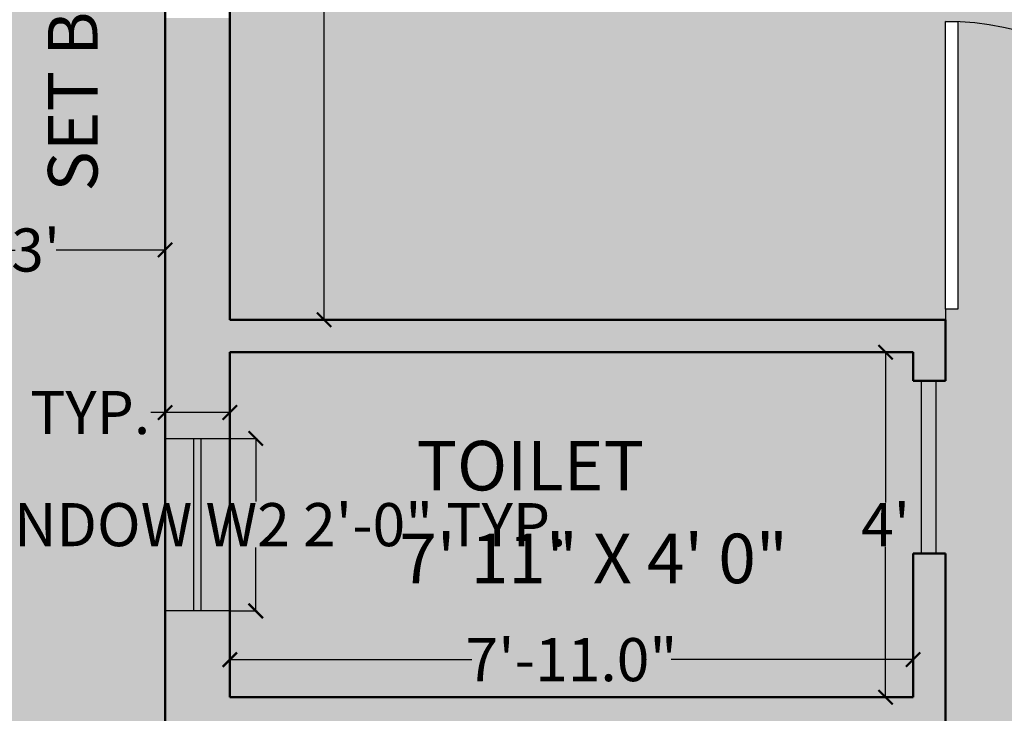
# Model space of a CAD drawing. Units: inches. Extents: x 528 to 2620, y -1066 to 798.
# Tile 6 of 41: x 600 to 737, y 523 to 620. Entities that reach past the tile are written whole.
import ezdxf

# ---------------------------------------------------------------- set-up
doc = ezdxf.new("R2010")
doc.units = ezdxf.units.IN
doc.header["$MEASUREMENT"] = 0
for name, color, linetype, lineweight in [('A-ANNO-DIMS', 2, 'Continuous', 18), ('A-AREA-IDEN', 7, 'Continuous', 18), ('A-Door', 2, 'Continuous', 25), ('A-GLAZ', 3, 'Continuous', 25), ('A-WALL', 7, 'Continuous', 50), ('A-WALL-PATT', 8, 'Continuous', 13)]:
    doc.layers.add(name, color=color, linetype=linetype, lineweight=lineweight)
doc.styles.get("Standard").update_dxf_attribs({"font": 'arial.ttf'})
doc.dimstyles.get("Standard").update_dxf_attribs({"dimtxt": 6, "dimasz": 2, "dimexe": 0.18, "dimexo": 0.0625, "dimgap": 0.09, "dimtad": 0, "dimtih": 1, "dimtoh": 1, "dimdec": 1, "dimzin": 0, "dimdsep": 46, "dimlunit": 3, "dimtxsty": 'Standard', "dimblk": 'ARCHTICK', "dimcen": 0.09, "dimadec": 0, "dimazin": 0, "dimtfac": 1, "dimtdec": 1, "dimtofl": 0, "dimtmove": 0, "dimatfit": 3, "dimfxl": 1, "dimtolj": 1, "dimtzin": 0, "dimarcsym": 0})

# ---------------------------------------------------------------- blocks, each defined once
blk = doc.blocks.new('*U4')
for p, q in [((0, 0), (0, -6)), ((40, 0), (40, -6))]:
    blk.add_line(p, q)
blk.add_lwpolyline([(0, 0), (0, 40), (1.75, 40), (1.75, 0)], close=True)
blk.add_arc((0, 0), 40, 0, 90)
blk = doc.blocks.new('_ArchTick')
at = {"color": 0, "linetype": 'ByBlock', "const_width": 0.15}
blk.add_lwpolyline([(-0.5, -0.5), (0.5, 0.5)], dxfattribs=at)
blk = doc.blocks.new('*D14')
at = {"layer": 'A-ANNO-DIMS', "color": 0, "lineweight": -2, "transparency": 16777216}
for p, q in [((584.06, 587.76), (584.06, 587.45)), ((584.06, 587.63), (599.21, 587.63)), ((620.06, 587.63), (604.91, 587.63)), ((620.06, 587.76), (620.06, 587.45))]:
    blk.add_line(p, q, dxfattribs=at)
at = {"layer": 'Defpoints', "color": 0, "transparency": 16777216}
for p in [(584.06, 587.82), (584.06, 587.63), (620.06, 587.82)]:
    blk.add_point(p, dxfattribs=at)
at = {"layer": 'A-ANNO-DIMS', "color": 0, "lineweight": -2, "transparency": 16777216, "xscale": 2, "yscale": 2, "zscale": 2, "rotation": 180}
blk.add_blockref('_ArchTick', (584.06, 587.63), dxfattribs=at)
at = {"layer": 'A-ANNO-DIMS', "color": 0, "lineweight": -2, "transparency": 16777216, "xscale": 2, "yscale": 2, "zscale": 2}
blk.add_blockref('_ArchTick', (620.06, 587.63), dxfattribs=at)
at = {"layer": 'A-ANNO-DIMS', "color": 0, "transparency": 16777216, "insert": (602.06, 587.63), "char_height": 6, "attachment_point": 5}
blk.add_mtext("\\A1;3'", dxfattribs=at)
blk = doc.blocks.new('*D26')
at = {"layer": 'A-ANNO-DIMS', "color": 0, "lineweight": -2, "transparency": 16777216}
for p, q in [((642.51, 709.92), (641.99, 709.92)), ((642.17, 709.92), (642.17, 647.02)), ((642.17, 577.92), (642.17, 640.82)), ((642.51, 577.92), (641.99, 577.92))]:
    blk.add_line(p, q, dxfattribs=at)
at = {"layer": 'Defpoints', "color": 0, "transparency": 16777216}
for p in [(642.57, 709.92), (642.17, 577.92), (642.57, 577.92)]:
    blk.add_point(p, dxfattribs=at)
at = {"layer": 'A-ANNO-DIMS', "color": 0, "lineweight": -2, "transparency": 16777216, "xscale": 2, "yscale": 2, "zscale": 2}
for p, rotation in [((642.17, 709.92), 90), ((642.17, 577.92), 270)]:
    blk.add_blockref('_ArchTick', p, dxfattribs=dict(at, rotation=rotation))
at = {"layer": 'A-ANNO-DIMS', "color": 0, "transparency": 16777216, "insert": (642.17, 643.92), "char_height": 6, "attachment_point": 5}
blk.add_mtext("\\A1;11'", dxfattribs=at)
blk = doc.blocks.new('*D31')
at = {"layer": 'A-ANNO-DIMS', "color": 0, "lineweight": -2, "transparency": 16777216}
for p, q in [((720.5, 573.42), (720.06, 573.42)), ((720.24, 573.42), (720.24, 552.51)), ((720.24, 525.42), (720.24, 546.33)), ((720.5, 525.42), (720.06, 525.42))]:
    blk.add_line(p, q, dxfattribs=at)
at = {"layer": 'Defpoints', "color": 0, "transparency": 16777216}
for p in [(720.56, 573.42), (720.24, 525.42), (720.56, 525.42)]:
    blk.add_point(p, dxfattribs=at)
at = {"layer": 'A-ANNO-DIMS', "color": 0, "lineweight": -2, "transparency": 16777216, "xscale": 2, "yscale": 2, "zscale": 2}
for p, rotation in [((720.24, 573.42), 90), ((720.24, 525.42), 270)]:
    blk.add_blockref('_ArchTick', p, dxfattribs=dict(at, rotation=rotation))
at = {"layer": 'A-ANNO-DIMS', "color": 0, "transparency": 16777216, "insert": (720.24, 549.42), "char_height": 6, "attachment_point": 5}
blk.add_mtext("\\A1;4'", dxfattribs=at)
blk = doc.blocks.new('*D32')
at = {"layer": 'A-ANNO-DIMS', "color": 0, "lineweight": -2, "transparency": 16777216}
for p, q in [((629.06, 530.64), (662.69, 530.64)), ((629.06, 530.58), (629.06, 530.46)), ((724.06, 530.64), (690.43, 530.64)), ((724.06, 530.7), (724.06, 530.82))]:
    blk.add_line(p, q, dxfattribs=at)
at = {"layer": 'Defpoints', "color": 0, "transparency": 16777216}
for p in [(629.06, 530.64), (724.06, 530.64), (724.06, 530.64)]:
    blk.add_point(p, dxfattribs=at)
at = {"layer": 'A-ANNO-DIMS', "color": 0, "lineweight": -2, "transparency": 16777216, "xscale": 2, "yscale": 2, "zscale": 2, "rotation": 180}
blk.add_blockref('_ArchTick', (629.06, 530.64), dxfattribs=at)
at = {"layer": 'A-ANNO-DIMS', "color": 0, "lineweight": -2, "transparency": 16777216, "xscale": 2, "yscale": 2, "zscale": 2}
blk.add_blockref('_ArchTick', (724.06, 530.64), dxfattribs=at)
at = {"layer": 'A-ANNO-DIMS', "color": 0, "transparency": 16777216, "insert": (676.56, 530.64), "char_height": 6, "attachment_point": 5}
blk.add_mtext('\\A1;7\'-11.0"', dxfattribs=at)
blk = doc.blocks.new('WIN-600')
for p, q in [((790.56, 714.92), (814.56, 714.92)), ((790.56, 713.92), (814.56, 713.92))]:
    blk.add_line(p, q)
blk.add_lwpolyline([(790.56, 718.92), (814.56, 718.92), (814.56, 709.92), (790.56, 709.92)], close=True)
blk = doc.blocks.new('*D52')
at = {"layer": 'A-ANNO-DIMS', "color": 0, "lineweight": -2, "transparency": 16777216}
for p, q in [((629.12, 561.42), (632.84, 561.42)), ((632.66, 561.42), (632.66, 552.62)), ((632.66, 537.42), (632.66, 546.23)), ((629.12, 537.42), (632.84, 537.42))]:
    blk.add_line(p, q, dxfattribs=at)
at = {"layer": 'Defpoints', "color": 0, "transparency": 16777216}
for p in [(629.06, 561.42), (632.66, 561.42), (629.06, 537.42)]:
    blk.add_point(p, dxfattribs=at)
at = {"layer": 'A-ANNO-DIMS', "color": 0, "lineweight": -2, "transparency": 16777216, "xscale": 2, "yscale": 2, "zscale": 2}
for p, rotation in [((632.66, 561.42), 90), ((632.66, 537.42), 270)]:
    blk.add_blockref('_ArchTick', p, dxfattribs=dict(at, rotation=rotation))
at = {"layer": 'A-ANNO-DIMS', "color": 0, "transparency": 16777216, "insert": (632.66, 549.42), "char_height": 6, "attachment_point": 5}
blk.add_mtext('\\A1;WINDOW W2 2\'-0" TYP.', dxfattribs=at)
blk = doc.blocks.new('*D53')
at = {"layer": 'A-ANNO-DIMS', "color": 0, "lineweight": -2, "transparency": 16777216}
for p, q in [((620.06, 565.02), (618.06, 565.02)), ((620.06, 561.48), (620.06, 565.2)), ((629.06, 565.02), (620.06, 565.02)), ((629.06, 561.48), (629.06, 565.2))]:
    blk.add_line(p, q, dxfattribs=at)
at = {"layer": 'Defpoints', "color": 0, "transparency": 16777216}
for p in [(620.06, 565.02), (620.06, 561.42), (629.06, 561.42)]:
    blk.add_point(p, dxfattribs=at)
at = {"layer": 'A-ANNO-DIMS', "color": 0, "lineweight": -2, "transparency": 16777216, "xscale": 2, "yscale": 2, "zscale": 2, "rotation": 180}
blk.add_blockref('_ArchTick', (620.06, 565.02), dxfattribs=at)
at = {"layer": 'A-ANNO-DIMS', "color": 0, "lineweight": -2, "transparency": 16777216, "xscale": 2, "yscale": 2, "zscale": 2}
blk.add_blockref('_ArchTick', (629.06, 565.02), dxfattribs=at)
at = {"layer": 'A-ANNO-DIMS', "color": 0, "transparency": 16777216, "insert": (599.68, 565.02), "char_height": 6, "attachment_point": 5}
blk.add_mtext('\\A1;0\'-9" TYP.', dxfattribs=at)

msp = doc.modelspace()

# ---------------------------------------------------------------- hatches: boundary and pattern name
at = {"layer": 'A-Door', "transparency": 33554521}
h = msp.add_hatch(color=256, dxfattribs=at)
h.dxf.hatch_style = 1
h.paths.add_polyline_path([(727.25, 569.42), (725.25, 569.42), (725.25, 545.42), (727.25, 545.42)])
at = {"layer": 'A-WALL-PATT', "transparency": 33554475}
h = msp.add_hatch(color=256, dxfattribs=at)
h.dxf.hatch_style = 1
h.paths.add_polyline_path([(620.06, 718.92), (908.06, 718.92), (908.06, 268.92), (770.06, 268.92), (770.06, 220.92), (932.06, 220.92), (932.06, 741.92), (596.06, 741.92), (596.06, 391.42), (620.06, 391.42)])
at = {"layer": 'A-WALL-PATT', "transparency": 33554687}
h = msp.add_hatch(color=256, dxfattribs=at)
h.dxf.hatch_style = 1
h.paths.add_polyline_path([(861.06, 273.92), (817.06, 273.92), (817.06, 272.92), (861.06, 272.92)])
h.paths.add_polyline_path([(817.06, 277.92), (815.06, 277.92), (815.06, 268.92), (817.06, 268.92)])
h.paths.add_polyline_path([(908.06, 397.92), (899.06, 397.92), (899.06, 395.92), (908.06, 395.92)])
h.paths.add_polyline_path([(908.06, 443.92), (899.06, 443.92), (899.06, 441.92), (908.06, 441.92)])
h.paths.add_polyline_path([(904.06, 441.92), (903.06, 441.92), (903.06, 397.92), (904.06, 397.92)])
h.paths.add_polyline_path([(625.06, 561.42), (624.06, 561.42), (624.06, 537.42), (625.06, 537.42)])
h.paths.add_polyline_path([(648.75, 334.44), (720.04, 334.44), (720.04, 345), (648.75, 345)], flags=9)
h.paths.add_polyline_path([(819.73, 323.15), (880.33, 323.15), (880.33, 333.71), (819.73, 333.71)], flags=9)
h.paths.add_polyline_path([(779.9, 680.61), (821.76, 680.61), (821.76, 691.17), (779.9, 691.17)], flags=9)
h.paths.add_polyline_path([(779.88, 692.36), (817.14, 692.36), (817.14, 703.06), (779.88, 703.06)], flags=9)
h.paths.add_polyline_path([(799.99, 453.88), (860.59, 453.88), (860.59, 464.44), (799.99, 464.44)], flags=9)
h.paths.add_polyline_path([(650.87, 539.4), (708.78, 539.4), (708.78, 549.95), (650.87, 549.95)], flags=9)
h.paths.add_polyline_path([(788.5, 612.01), (849.1, 612.01), (849.1, 622.56), (788.5, 622.56)], flags=9)
h.paths.add_polyline_path([(639.54, 648.31), (700.13, 648.31), (700.13, 658.87), (639.54, 658.87)], flags=9)
h.paths.add_polyline_path([(648.91, 346.09), (747.71, 346.09), (747.71, 356.78), (648.91, 356.78)], flags=9)
h.paths.add_polyline_path([(676.86, 450.66), (746.74, 450.66), (746.74, 461.36), (676.86, 461.36)], flags=9)
h.paths.add_polyline_path([(819.71, 334.95), (865.53, 334.95), (865.53, 345.64), (819.71, 345.64)], flags=9)
h.paths.add_polyline_path([(806.3, 467.75), (874.05, 467.75), (874.05, 478.44), (806.3, 478.44)], flags=9)
h.paths.add_polyline_path([(653.23, 552.28), (690.5, 552.28), (690.5, 562.98), (653.23, 562.98)], flags=9)
h.paths.add_polyline_path([(789.9, 623.41), (843.21, 623.41), (843.21, 634.1), (789.9, 634.1)], flags=9)
h.paths.add_polyline_path([(639.77, 662.1), (693.08, 662.1), (693.08, 672.8), (639.77, 672.8)], flags=9)
h.paths.add_polyline_path([(801.59, 242.91), (846.33, 242.91), (846.33, 253.6), (801.59, 253.6)], flags=9)
h.paths.add_polyline_path([(925.36, 593.98), (925.36, 674.06), (914.67, 674.06), (914.67, 593.98)], flags=9)
h.paths.add_polyline_path([(612.56, 593.98), (612.56, 674.06), (601.87, 674.06), (601.87, 593.98)], flags=9)
h.paths.add_polyline_path([(723.31, 726.56), (803.39, 726.56), (803.39, 737.25), (723.31, 737.25)], flags=9)
at = {"layer": 'A-WALL-PATT', "transparency": 33554521}
h = msp.add_hatch(color=256, dxfattribs=at)
h.dxf.hatch_style = 1
h.paths.add_polyline_path([(629.06, 709.92), (677.56, 709.92), (677.56, 718.92), (620.06, 718.92), (620.06, 667.92), (629.06, 667.92)])
h.paths.add_polyline_path([(790.56, 718.92), (725.56, 718.92), (725.56, 709.92), (774.06, 709.92), (774.06, 577.92), (768.48, 577.92), (768.56, 573.42), (774.06, 573.42), (774.06, 567.42), (778.56, 567.42), (778.56, 669.42), (831.06, 669.42), (831.06, 675.92), (826.56, 675.92), (826.56, 673.92), (778.56, 673.92), (778.56, 709.92), (790.56, 709.92)])
h.paths.add_polyline_path([(908.06, 718.92), (879.06, 718.92), (879.06, 709.92), (899.06, 709.92), (899.06, 641.67), (908.06, 641.67)])
h.paths.add_polyline_path([(629.06, 619.92), (620.06, 619.92), (620.06, 561.42), (629.06, 561.42), (629.06, 573.42), (724.06, 573.42), (724.06, 569.42), (728.56, 569.42), (728.56, 577.92), (629.06, 577.92)])
h.paths.add_polyline_path([(779.06, 391.42), (779.06, 400.42), (770.06, 400.42), (764.06, 400.42), (764.06, 397.42), (764.06, 391.42), (770.06, 391.42), (770.06, 268.92), (815.06, 268.92), (815.06, 277.92), (779.06, 277.92), (779.06, 359.77)])
h.paths.add_polyline_path([(908.06, 395.92), (899.06, 395.92), (851.06, 395.92), (851.06, 391.42), (899.06, 391.42), (899.06, 277.92), (863.06, 277.92), (863.06, 268.92), (908.06, 268.92)])
h.paths.add_polyline_path([(908.06, 593.67), (899.06, 593.67), (899.06, 525.42), (778.56, 525.42), (778.56, 527.17), (774.06, 527.17), (774.06, 520.92), (899.06, 520.92), (899.06, 443.92), (908.06, 443.92)])
h.paths.add_polyline_path([(629.06, 520.92), (728.56, 520.92), (728.56, 545.42), (724.06, 545.42), (724.06, 525.42), (629.06, 525.42), (629.06, 537.42), (620.06, 537.42), (620.06, 484.67), (629.06, 484.67)])
h.paths.add_polyline_path([(629.06, 436.67), (620.06, 436.67), (620.06, 391.42), (648.56, 391.42), (648.56, 400.42), (629.06, 400.42)])
h.paths.add_polyline_path([(716.06, 397.42), (716.06, 400.42), (696.56, 400.42), (696.56, 391.42), (716.06, 391.42)])
at = {"layer": 'A-WALL-PATT', "transparency": 33554681}
h = msp.add_hatch(color=256, dxfattribs=at)
h.dxf.hatch_style = 1
h.paths.add_polyline_path([(629.06, 665.92), (625.06, 665.92), (625.06, 621.92), (629.06, 621.92)])
h.paths.add_polyline_path([(624.06, 665.92), (620.06, 665.92), (620.06, 621.92), (624.06, 621.92)])
h.paths.add_polyline_path([(723.56, 713.92), (679.56, 713.92), (679.56, 709.92), (723.56, 709.92)])
h.paths.add_polyline_path([(723.56, 718.92), (679.56, 718.92), (679.56, 714.92), (723.56, 714.92)])
h.paths.add_polyline_path([(814.56, 713.92), (790.56, 713.92), (790.56, 709.92), (814.56, 709.92)])
h.paths.add_polyline_path([(814.56, 718.92), (790.56, 718.92), (790.56, 714.92), (814.56, 714.92)])
h.paths.add_polyline_path([(877.06, 713.92), (833.06, 713.92), (833.06, 709.92), (877.06, 709.92)])
h.paths.add_polyline_path([(877.06, 718.92), (833.06, 718.92), (833.06, 714.92), (877.06, 714.92)])
h.paths.add_polyline_path([(908.06, 639.67), (904.06, 639.67), (904.06, 595.67), (908.06, 595.67)])
h.paths.add_polyline_path([(903.06, 639.67), (899.06, 639.67), (899.06, 595.67), (903.06, 595.67)])
h.paths.add_polyline_path([(908.06, 441.92), (904.06, 441.92), (904.06, 397.92), (908.06, 397.92)])
h.paths.add_polyline_path([(903.06, 441.92), (899.06, 441.92), (899.06, 397.92), (903.06, 397.92)])
h.paths.add_polyline_path([(861.06, 272.92), (817.06, 272.92), (817.06, 268.92), (861.06, 268.92)])
h.paths.add_polyline_path([(861.06, 277.92), (817.06, 277.92), (817.06, 273.92), (861.06, 273.92)])
h.paths.add_polyline_path([(694.56, 395.42), (650.56, 395.42), (650.56, 391.42), (694.56, 391.42)])
h.paths.add_polyline_path([(694.56, 400.42), (650.56, 400.42), (650.56, 396.42), (694.56, 396.42)])
h.paths.add_polyline_path([(629.06, 482.67), (625.06, 482.67), (625.06, 438.67), (629.06, 438.67)])
h.paths.add_polyline_path([(624.06, 482.67), (620.06, 482.67), (620.06, 438.67), (624.06, 438.67)])
h.paths.add_polyline_path([(629.06, 561.42), (625.06, 561.42), (625.06, 537.42), (629.06, 537.42)])
h.paths.add_polyline_path([(624.06, 561.42), (620.06, 561.42), (620.06, 537.42), (624.06, 537.42)])
at = {"layer": 'A-WALL-PATT', "transparency": 33554590}
h = msp.add_hatch(color=256, dxfattribs=at)
h.dxf.hatch_style = 1
h.paths.add_polyline_path([(774.06, 709.92), (629.06, 709.92), (629.06, 577.92), (728.56, 577.92), (728.56, 579.42), (728.56, 619.42), (730.31, 619.42), (730.31, 619.38, -0.401453), (768.56, 579.42), (768.56, 577.92), (774.06, 577.92)])
h.paths.add_polyline_path([(723.9, 686.06), (723.97, 686.06), (723.83, 686.13)], flags=0)
h.paths.add_polyline_path([(722.79, 642.7), (722.89, 642.76), (722.89, 684.99), (722.65, 685.24), (722.65, 685.82), (723.08, 686.26), (723.53, 686.26), (723.97, 686.06), (724.74, 686.13), (770.7, 686.13), (770.78, 686.14), (771.13, 686.27), (771.69, 686.09), (771.94, 685.48), (771.67, 684.9), (771.58, 684.87), (771.58, 642.78), (771.88, 642.51), (771.88, 641.92), (771.51, 641.46), (770.85, 641.46), (770.4, 641.83), (770.4, 641.55), (724.74, 641.55), (723.99, 641.7), (723.44, 641.41), (722.88, 641.59), (722.6, 642.14)], flags=16)
h.paths.add_polyline_path([(723.99, 641.7), (723.99, 641.71), (723.99, 641.7)], flags=0)
h.paths.add_polyline_path([(722.89, 642.73), (722.89, 684.99), (722.65, 685.24), (722.65, 685.82), (723.08, 686.26), (723.29, 686.26), (722.99, 686.17), (722.79, 685.97), (722.65, 685.68), (722.65, 685.43), (722.75, 685.14), (722.94, 684.94), (723.24, 684.81), (723.48, 684.81), (723.78, 684.9), (723.98, 685.1), (724.17, 685.49), (724.12, 685.64), (724.12, 685.25), (723.63, 684.75), (723.63, 642.96), (724.12, 642.51), (724.12, 641.89), (723.66, 641.46), (723.08, 641.46), (722.65, 641.9), (722.65, 642.48)], flags=0)
h.paths.add_polyline_path([(722.65, 642.29), (722.65, 642.04), (722.79, 641.75), (723.08, 641.46), (723.29, 641.46), (722.88, 641.59), (722.6, 642.14)], flags=0)
h.paths.add_polyline_path([(770.75, 686.13), (770.58, 686.13), (770.55, 686.06)], flags=0)
h.paths.add_polyline_path([(743.3, 645.29), (753.23, 659.4), (748.69, 663.75), (753.23, 668.54), (743.3, 682.46), (743.79, 682.59), (744.14, 682.68), (744.53, 682.93), (744.63, 683.08), (745.02, 683.33), (744.53, 684.07), (744.78, 684.16), (744.87, 684.31), (745.51, 684.4), (746.08, 684.65), (746.47, 684.65), (746.82, 684.81), (747.46, 685.03), (747.71, 685.14), (748.2, 685.28), (748.39, 685.52), (748.86, 685.52), (749.99, 686.13), (753.49, 676.03), (757.38, 680.15), (757.79, 679.76), (758.04, 680.65), (758.29, 681.23), (758.29, 682.05), (758.02, 682.59), (757.87, 683.17), (757.82, 683.78), (758.39, 684.07), (758.98, 684.2), (759.62, 684.16), (760.21, 683.96), (760.75, 683.67), (761.86, 683.67), (762.4, 683.96), (762.99, 684.11), (763.63, 684.11), (764.2, 683.96), (764.74, 683.67), (766.12, 683.67), (766.66, 683.96), (767.25, 684.16), (767.87, 684.2), (768.46, 684.07), (769.05, 683.78), (769, 683.17), (768.85, 682.59), (768.55, 682.05), (768.55, 681.23), (768.8, 680.65), (769.09, 679.75), (768.95, 678.83), (768.8, 678.23), (768.55, 677.65), (768.55, 676.82), (768.8, 676.24), (769.09, 675.34), (768.95, 674.42), (768.8, 673.82), (768.55, 673.28), (768.55, 672.41), (768.8, 671.87), (769, 671.29), (769.05, 670.64), (768.95, 670.02), (768.8, 669.41), (768.55, 668.87), (768.55, 668), (768.97, 667.24), (769.05, 666.28), (769.05, 665.56), (768.46, 665.32), (767.87, 665.16), (767.25, 665.16), (766.66, 665.36), (766.12, 665.7), (764.74, 665.7), (763.94, 665.2), (762.99, 665.2), (762.4, 665.36), (761.86, 665.7), (761, 665.7), (762.7, 664.09), (760.74, 662.03), (761.86, 662.03), (762.4, 662.32), (763.34, 662.55), (764.25, 662.32), (764.79, 662.03), (766.12, 662.03), (766.66, 662.32), (767.25, 662.52), (767.87, 662.56), (768.51, 662.43), (769.05, 662.12), (769.05, 661.4), (769.05, 660.8), (768.85, 660.21), (768.55, 659.68), (768.55, 658.85), (768.85, 658.27), (769, 657.66), (769.07, 656.75), (768.85, 655.85), (768.55, 655.27), (768.55, 654.44), (768.85, 653.86), (769.07, 652.96), (769, 652.05), (768.85, 651.44), (768.55, 650.91), (768.55, 650.03), (768.85, 649.5), (769, 648.91), (769.05, 648.26), (769, 647.64), (768.85, 647.03), (768.55, 646.5), (768.55, 645.62), (768.85, 645.09), (769.05, 644.55), (769.05, 643.9), (768.51, 643.65), (767.87, 643.52), (767.25, 643.52), (766.66, 643.72), (766.12, 644.06), (764.79, 644.06), (764.25, 643.72), (763.34, 643.49), (762.4, 643.72), (761.86, 644.06), (760.8, 644.06), (760.26, 643.72), (759.67, 643.52), (759.03, 643.52), (758.39, 643.65), (757.87, 643.9), (757.87, 644.55), (758.04, 645.09), (758.34, 645.62), (758.34, 646.5), (758.04, 647.03), (757.92, 647.64), (757.87, 648.06), (757.38, 647.59), (753.42, 651.77), (749.99, 641.62), (749.5, 641.71), (749.35, 641.95), (748.54, 642.45), (747.31, 642.94), (746.65, 642.94), (746.33, 643.18), (745.51, 643.57), (744.53, 643.65), (745.01, 644.4), (744.63, 644.64), (744.14, 644.89), (743.79, 645.13)], flags=0)
h.paths.add_polyline_path([(755.66, 654.93), (756.54, 654.69), (757.53, 654.33), (756.64, 654.58)], flags=0)
h.paths.add_polyline_path([(758.34, 649.2), (758.34, 648.71), (758.59, 644.3), (758.59, 648.8)], flags=0)
h.paths.add_polyline_path([(758.34, 649.29), (758.09, 649.7), (758.36, 649.17)], flags=0)
h.paths.add_polyline_path([(755.66, 672.79), (756.49, 673.04), (757.36, 673.35), (757.35, 673.36), (756.64, 673.15)], flags=0)
h.paths.add_polyline_path([(760.26, 639.64), (771.41, 639.64), (771.41, 624.04), (760.26, 624.04)], flags=16)
h.paths.add_polyline_path([(761.38, 638.53), (770.29, 638.53), (770.29, 625.15), (761.38, 625.15)], flags=0)
edge = h.paths.add_edge_path(flags=0)
edge.add_ellipse((765.84, 631.84), major_axis=(-2.24, 2.24), ratio=1, start_angle=-45, end_angle=45, ccw=False)
edge.add_ellipse((765.84, 631.84), major_axis=(-2.24, 2.24), ratio=1, start_angle=-135, end_angle=-45, ccw=False)
edge.add_ellipse((765.84, 631.84), major_axis=(-2.24, 2.24), ratio=1, start_angle=135, end_angle=-135, ccw=False)
edge.add_ellipse((765.84, 631.84), major_axis=(-2.24, 2.24), ratio=1, start_angle=45, end_angle=135, ccw=False)
h.paths.add_polyline_path([(758.59, 683.42), (758.59, 678.92), (758.37, 678.58), (758.34, 678.43), (758.09, 678.05), (758.34, 678.52), (758.34, 679.01)], flags=0)
h.paths.add_polyline_path([(760.26, 688.04), (760.26, 703.64), (771.41, 703.64), (771.41, 688.04)], flags=16)
h.paths.add_polyline_path([(770.4, 685.39), (770.4, 685.85), (770.85, 686.22), (771.51, 686.22), (771.88, 685.76), (771.88, 685.17), (771.58, 684.9), (771.58, 642.78), (771.88, 642.51), (771.88, 641.92), (771.51, 641.46), (770.85, 641.46), (770.4, 641.83), (770.4, 642.29)], flags=0)
h.paths.add_polyline_path([(770.53, 642.68), (771.05, 643.01), (771.67, 642.77), (771.94, 642.2), (771.69, 641.59), (771.13, 641.41), (770.55, 641.62), (770.35, 642.13)], flags=16)
h.paths.add_polyline_path([(761.38, 689.15), (761.38, 702.53), (770.29, 702.53), (770.29, 689.15)], flags=0)
edge = h.paths.add_edge_path(flags=0)
edge.add_ellipse((765.84, 695.84), major_axis=(2.24, 2.24), ratio=1, start_angle=405, end_angle=495, ccw=False)
edge.add_ellipse((765.84, 695.84), major_axis=(2.24, 2.24), ratio=1, start_angle=675, end_angle=765, ccw=False)
edge.add_ellipse((765.84, 695.84), major_axis=(2.24, 2.24), ratio=1, start_angle=585, end_angle=675, ccw=False)
edge.add_ellipse((765.84, 695.84), major_axis=(2.24, 2.24), ratio=1, start_angle=495, end_angle=585, ccw=False)
h.paths.add_polyline_path([(770.7, 684.9), (770.94, 684.74), (771.41, 684.74), (771.73, 685.03), (771.88, 685.34), (771.88, 685.64), (771.69, 686.09), (771.58, 686.13), (771.88, 685.76), (771.88, 685.17), (771.41, 684.74), (770.85, 684.74)], flags=0)
h.paths.add_polyline_path([(899.06, 709.92), (831.06, 709.92), (831.06, 699.92), (829.81, 699.92), (829.81, 675.92), (831.06, 675.92), (831.06, 669.42), (778.56, 669.42), (778.56, 567.17), (780.06, 567.17), (820.06, 567.17), (820.06, 565.42), (820.02, 565.42, -0.401453), (780.06, 527.17), (778.56, 527.17), (778.56, 525.42), (899.06, 525.42)])
h.paths.add_polyline_path([(849.2, 636.01), (849.27, 636.02), (849.13, 636.08)], flags=0)
h.paths.add_polyline_path([(848.19, 634.95), (847.95, 635.2), (847.95, 635.78), (848.38, 636.22), (848.83, 636.22), (849.27, 636.02), (850.04, 636.08), (896, 636.08), (896.08, 636.1), (896.43, 636.22), (896.99, 636.05), (897.24, 635.43), (896.97, 634.86), (896.88, 634.83), (896.88, 592.74), (897.18, 592.47), (897.18, 591.88), (896.81, 591.42), (896.15, 591.42), (895.7, 591.79), (895.7, 591.51), (850.04, 591.51), (849.29, 591.66), (848.74, 591.37), (848.18, 591.54), (847.9, 592.1), (848.09, 592.65), (848.19, 592.71)], flags=16)
h.paths.add_polyline_path([(849.29, 591.66), (849.29, 591.66), (849.29, 591.66)], flags=16)
h.paths.add_polyline_path([(848.19, 634.95), (847.95, 635.2), (847.95, 635.78), (848.38, 636.22), (848.59, 636.22), (848.29, 636.13), (848.09, 635.93), (847.95, 635.64), (847.95, 635.39), (848.05, 635.1), (848.24, 634.9), (848.54, 634.76), (848.78, 634.76), (849.08, 634.85), (849.28, 635.05), (849.47, 635.44), (849.42, 635.59), (849.42, 635.21), (848.93, 634.7), (848.93, 592.92), (849.42, 592.47), (849.42, 591.84), (848.96, 591.42), (848.38, 591.42), (847.95, 591.86), (847.95, 592.44), (848.19, 592.69)], flags=0)
h.paths.add_polyline_path([(847.95, 592.25), (847.95, 592), (848.09, 591.71), (848.38, 591.42), (848.59, 591.42), (848.18, 591.54), (847.9, 592.1)], flags=16)
h.paths.add_polyline_path([(896.05, 636.08), (895.88, 636.08), (895.85, 636.01)], flags=0)
h.paths.add_polyline_path([(868.6, 632.41), (869.09, 632.55), (869.44, 632.64), (869.83, 632.88), (869.93, 633.04), (870.32, 633.28), (869.83, 634.02), (870.08, 634.11), (870.17, 634.27), (870.81, 634.36), (871.38, 634.61), (871.77, 634.61), (872.12, 634.76), (872.76, 634.99), (873.01, 635.1), (873.5, 635.23), (873.69, 635.48), (874.16, 635.48), (875.29, 636.08), (878.79, 625.99), (882.68, 630.11), (883.09, 629.71), (883.34, 630.6), (883.59, 631.18), (883.59, 632.01), (883.32, 632.55), (883.17, 633.13), (883.12, 633.73), (883.69, 634.02), (884.28, 634.16), (884.92, 634.11), (885.51, 633.91), (886.05, 633.62), (887.16, 633.62), (887.7, 633.91), (888.29, 634.07), (888.93, 634.07), (889.5, 633.91), (890.04, 633.62), (891.42, 633.62), (891.96, 633.91), (892.55, 634.11), (893.17, 634.16), (893.76, 634.02), (894.35, 633.73), (894.3, 633.13), (894.15, 632.55), (893.85, 632.01), (893.85, 631.18), (894.1, 630.6), (894.39, 629.71), (894.25, 628.79), (894.1, 628.18), (893.85, 627.6), (893.85, 626.77), (894.1, 626.19), (894.39, 625.3), (894.25, 624.38), (894.1, 623.78), (893.85, 623.24), (893.85, 622.37), (894.1, 621.83), (894.3, 621.25), (894.35, 620.6), (894.25, 619.97), (894.1, 619.37), (893.85, 618.83), (893.85, 617.96), (894.27, 617.2), (894.35, 616.23), (894.35, 615.52), (893.76, 615.27), (893.17, 615.12), (892.55, 615.12), (891.96, 615.32), (891.42, 615.65), (890.04, 615.65), (889.25, 615.16), (888.29, 615.16), (887.7, 615.32), (887.16, 615.65), (886.31, 615.65), (888, 614.04), (886.04, 611.98), (887.16, 611.98), (887.7, 612.27), (888.64, 612.5), (889.55, 612.27), (890.09, 611.98), (891.42, 611.98), (891.96, 612.27), (892.55, 612.48), (893.17, 612.52), (893.81, 612.39), (894.35, 612.07), (894.35, 611.36), (894.35, 610.75), (894.15, 610.17), (893.85, 609.63), (893.85, 608.81), (894.15, 608.22), (894.3, 607.62), (894.37, 606.7), (894.15, 605.81), (893.85, 605.22), (893.85, 604.4), (894.15, 603.81), (894.37, 602.92), (894.3, 602), (894.15, 601.4), (893.85, 600.86), (893.85, 599.99), (894.15, 599.45), (894.3, 598.87), (894.35, 598.22), (894.3, 597.59), (894.15, 596.99), (893.85, 596.45), (893.85, 595.58), (894.15, 595.04), (894.35, 594.51), (894.35, 593.86), (893.81, 593.61), (893.17, 593.48), (892.55, 593.48), (891.96, 593.68), (891.42, 594.01), (890.09, 594.01), (889.55, 593.68), (888.64, 593.45), (887.7, 593.68), (887.16, 594.01), (886.1, 594.01), (885.56, 593.68), (884.97, 593.48), (884.33, 593.48), (883.69, 593.61), (883.17, 593.86), (883.17, 594.51), (883.34, 595.04), (883.64, 595.58), (883.64, 596.45), (883.34, 596.99), (883.22, 597.59), (883.17, 598.01), (882.68, 597.55), (878.72, 601.73), (875.29, 591.57), (874.8, 591.66), (874.65, 591.91), (873.84, 592.4), (872.61, 592.89), (871.95, 592.89), (871.63, 593.14), (870.81, 593.52), (869.83, 593.61), (870.31, 594.36), (869.93, 594.6), (869.44, 594.84), (869.09, 595.09), (868.6, 595.24), (878.53, 609.35), (873.99, 613.71), (878.53, 618.49)], flags=0)
h.paths.add_polyline_path([(880.96, 622.75), (881.79, 622.99), (882.66, 623.31), (882.65, 623.31), (881.94, 623.1)], flags=0)
h.paths.add_polyline_path([(880.96, 604.89), (881.84, 604.64), (882.83, 604.28), (881.94, 604.53)], flags=16)
h.paths.add_polyline_path([(883.39, 628.01), (883.64, 628.48), (883.64, 628.97), (883.89, 633.38), (883.89, 628.88), (883.67, 628.53), (883.64, 628.39)], flags=0)
h.paths.add_polyline_path([(883.64, 599.16), (883.64, 598.67), (883.89, 594.26), (883.89, 598.76)], flags=16)
h.paths.add_polyline_path([(883.64, 599.25), (883.39, 599.65), (883.66, 599.12)], flags=16)
h.paths.add_polyline_path([(885.56, 637.99), (885.56, 653.6), (896.71, 653.6), (896.71, 637.99)], flags=16)
h.paths.add_polyline_path([(885.56, 589.6), (896.71, 589.6), (896.71, 573.99), (885.56, 573.99)], flags=16)
h.paths.add_polyline_path([(886.68, 639.11), (886.68, 652.48), (895.59, 652.48), (895.59, 639.11)], flags=0)
h.paths.add_polyline_path([(886.68, 588.48), (895.59, 588.48), (895.59, 575.11), (886.68, 575.11)], flags=0)
edge = h.paths.add_edge_path(flags=0)
edge.add_ellipse((891.14, 645.79), major_axis=(2.24, 2.24), ratio=1, start_angle=405, end_angle=495, ccw=False)
edge.add_ellipse((891.14, 645.79), major_axis=(2.24, 2.24), ratio=1, start_angle=675, end_angle=765, ccw=False)
edge.add_ellipse((891.14, 645.79), major_axis=(2.24, 2.24), ratio=1, start_angle=585, end_angle=675, ccw=False)
edge.add_ellipse((891.14, 645.79), major_axis=(2.24, 2.24), ratio=1, start_angle=495, end_angle=585, ccw=False)
edge = h.paths.add_edge_path(flags=0)
edge.add_ellipse((891.14, 581.8), major_axis=(-2.24, 2.24), ratio=1, start_angle=-45, end_angle=45, ccw=False)
edge.add_ellipse((891.14, 581.8), major_axis=(-2.24, 2.24), ratio=1, start_angle=-135, end_angle=-45, ccw=False)
edge.add_ellipse((891.14, 581.8), major_axis=(-2.24, 2.24), ratio=1, start_angle=135, end_angle=-135, ccw=False)
edge.add_ellipse((891.14, 581.8), major_axis=(-2.24, 2.24), ratio=1, start_angle=45, end_angle=135, ccw=False)
h.paths.add_polyline_path([(895.7, 635.35), (895.7, 635.8), (896.15, 636.17), (896.81, 636.17), (897.18, 635.71), (897.18, 635.12), (896.88, 634.85), (896.88, 592.74), (897.18, 592.47), (897.18, 591.88), (896.81, 591.42), (896.15, 591.42), (895.7, 591.79), (895.7, 592.25)], flags=0)
h.paths.add_polyline_path([(896, 634.85), (896.24, 634.7), (896.71, 634.7), (897.03, 634.99), (897.18, 635.3), (897.18, 635.59), (896.99, 636.05), (896.88, 636.08), (897.18, 635.71), (897.18, 635.12), (896.71, 634.7), (896.15, 634.7)], flags=0)
h.paths.add_polyline_path([(895.83, 592.63), (896.35, 592.96), (896.97, 592.73), (897.24, 592.16), (896.99, 591.54), (896.43, 591.37), (895.85, 591.58), (895.65, 592.09)], flags=16)
h.paths.add_polyline_path([(725.25, 569.42), (724.06, 569.42), (724.06, 573.42), (629.06, 573.42), (629.06, 525.42), (724.06, 525.42), (724.06, 545.42), (725.25, 545.42)])
h.paths.add_polyline_path([(820.02, 565.42), (780.06, 565.42), (780.06, 567.17), (774.06, 567.17), (774.06, 567.42), (774.06, 573.42), (768.56, 573.42), (768.48, 577.92), (768.56, 577.92), (768.56, 579.42, 0.401453), (730.31, 619.38), (730.31, 579.42), (728.56, 579.42), (728.56, 573.42), (728.56, 569.42), (727.25, 569.42), (727.25, 545.42), (728.56, 545.42), (728.56, 520.92), (665.06, 520.92), (665.06, 436.42), (716.06, 436.42), (716.06, 421.42), (717.81, 421.42), (717.81, 421.36, -0.392996), (740.06, 397.42, -0.392996), (762.31, 421.36), (762.31, 421.42), (764.06, 421.42), (764.06, 400.42), (770.06, 400.42), (779.06, 400.42), (779.06, 391.42), (779.06, 359.77), (795.43, 359.77), (795.43, 294.3), (893.67, 294.3), (893.67, 277.92), (899.06, 277.92), (899.06, 391.42), (851.06, 391.42), (851.06, 395.92), (899.06, 395.92), (899.06, 443.92), (899.06, 520.92), (774.06, 520.92), (774.06, 527.17), (778.56, 527.17), (780.06, 527.17, 0.401453)])
h.paths.add_polyline_path([(774.06, 519.66), (842.12, 519.66), (842.12, 505.07), (788.64, 505.07), (788.64, 474.08), (788.64, 470.43, -0.883215), (779.53, 456.66), (774.97, 456.66, -0.414214), (774.06, 457.57)], flags=16)
h.paths.add_polyline_path([(775.88, 517.83), (840.3, 517.83), (840.3, 514.19), (788.64, 514.19), (788.64, 484.41), (779.53, 484.41), (779.53, 474.08), (775.88, 474.08)], flags=0)
h.paths.add_polyline_path([(706.7, 501.56, -0.254069), (706.7, 493.02), (698.31, 492.55), (698.31, 502.03)], flags=16)
h.paths.add_polyline_path([(691.33, 515.69), (691.8, 507.3), (682.32, 507.3), (682.79, 515.69, -0.254069)], flags=16)
h.paths.add_polyline_path([(695.49, 504.68), (695.49, 479.42), (678.64, 479.42), (678.64, 504.68)], flags=16)
h.paths.add_polyline_path([(706.7, 489.6, -0.254069), (706.7, 481.06), (698.31, 480.59), (698.31, 490.07)], flags=16)
h.paths.add_polyline_path([(675.81, 502.03), (675.81, 492.55), (667.42, 493.02, -0.254069), (667.42, 501.56)], flags=16)
h.paths.add_polyline_path([(691.8, 476.8), (691.33, 468.41, -0.254069), (682.79, 468.41), (682.32, 476.8)], flags=16)
h.paths.add_polyline_path([(675.81, 490.07), (675.81, 480.59), (667.42, 481.06, -0.254069), (667.42, 489.6)], flags=16)
h.paths.add_polyline_path([(764.06, 397.42), (762.31, 397.42), (762.31, 421.36, 0.392996), (740.06, 397.42, 0.392996), (717.81, 421.36), (717.81, 397.42), (716.06, 397.42), (716.06, 391.42), (716.06, 385.42), (764.06, 385.42), (764.06, 391.42)], flags=17)
h.paths.add_polyline_path([(716.06, 436.42), (705.86, 436.42), (705.86, 418.42), (716.06, 418.42), (716.06, 421.42)], flags=17)
h.paths.add_polyline_path([(716.06, 418.42), (705.86, 418.42), (705.86, 400.42), (716.06, 400.42)], flags=17)
h.paths.add_polyline_path([(705.86, 418.42), (695.66, 418.42), (695.66, 400.42), (696.56, 400.42), (705.86, 400.42)], flags=17)
h.paths.add_polyline_path([(705.86, 436.42), (695.66, 436.42), (695.66, 418.42), (705.86, 418.42)], flags=17)
h.paths.add_polyline_path([(695.66, 418.42), (685.46, 418.42), (685.46, 400.42), (695.66, 400.42)], flags=17)
h.paths.add_polyline_path([(695.66, 436.42), (685.46, 436.42), (685.46, 418.42), (695.66, 418.42)], flags=17)
h.paths.add_polyline_path([(685.46, 418.42), (675.26, 418.42), (675.26, 400.42), (685.46, 400.42)], flags=17)
h.paths.add_polyline_path([(685.46, 436.42), (675.26, 436.42), (675.26, 418.42), (685.46, 418.42)], flags=17)
h.paths.add_polyline_path([(675.26, 436.42), (665.06, 436.42), (665.06, 418.42), (675.26, 418.42)])
h.paths.add_polyline_path([(675.26, 418.42), (665.06, 418.42), (665.06, 400.42), (675.26, 400.42)])
h.paths.add_polyline_path([(665.06, 418.42), (646.97, 418.42), (646.99, 436.42), (629.06, 436.42), (629.06, 400.42), (665.06, 400.42)])
h.paths.add_polyline_path([(665.06, 436.42), (646.99, 436.42), (646.97, 418.42), (665.06, 418.42)], flags=17)
h.paths.add_polyline_path([(647.01, 446.62), (629.06, 446.62), (629.06, 436.67), (629.06, 436.42), (646.99, 436.42)])
h.paths.add_polyline_path([(665.06, 446.62), (647.01, 446.62), (646.99, 436.42), (665.06, 436.42)])
h.paths.add_polyline_path([(647.02, 456.82), (629.06, 456.82), (629.06, 446.62), (647.01, 446.62)])
h.paths.add_polyline_path([(665.06, 456.82), (647.02, 456.82), (647.01, 446.62), (665.06, 446.62)])
h.paths.add_polyline_path([(647.03, 467.02), (629.06, 467.02), (629.06, 456.82), (647.02, 456.82)])
h.paths.add_polyline_path([(665.06, 467.02), (647.03, 467.02), (647.02, 456.82), (665.06, 456.82)])
h.paths.add_polyline_path([(665.06, 477.22), (647.05, 477.22), (647.03, 467.02), (665.06, 467.02)])
h.paths.add_polyline_path([(647.05, 477.22), (629.06, 477.22), (629.06, 467.02), (647.03, 467.02)])
h.paths.add_polyline_path([(647.06, 487.22), (629.06, 487.22), (629.06, 477.22), (647.05, 477.22), (647.05, 479.02), (645.53, 483.25), (640.88, 480.37)])
h.paths.add_polyline_path([(665.06, 520.92), (629.06, 520.92), (629.06, 487.22), (647.06, 487.22), (665.06, 487.22)])
h.paths.add_polyline_path([(665.06, 487.22), (647.06, 487.22), (653.22, 480.35), (648.58, 483.24), (647.05, 479.02), (647.05, 477.22), (665.06, 477.22)])

# ---------------------------------------------------------------- linework, layer by layer
at = {"layer": 'A-Door'}
msp.add_lwpolyline([(727.25, 545.42), (725.25, 545.42), (725.25, 569.42), (727.25, 569.42)], close=True, dxfattribs=at)
at = {"layer": 'A-WALL'}
for p, q in [((620.06, 718.92), (620.06, 391.42)), ((629.06, 709.92), (629.06, 577.92)), ((728.56, 577.92), (629.06, 577.92)), ((728.56, 577.92), (728.56, 569.42)), ((629.06, 573.42), (629.06, 525.42)), ((724.06, 573.42), (629.06, 573.42)), ((724.06, 573.42), (724.06, 569.42)), ((724.06, 569.42), (728.56, 569.42)), ((724.06, 545.42), (728.56, 545.42)), ((724.06, 545.42), (724.06, 525.42)), ((728.56, 545.42), (728.56, 520.92)), ((724.06, 525.42), (629.06, 525.42))]:
    msp.add_line(p, q, dxfattribs=at)

# ---------------------------------------------------------------- block references
at = {"layer": 'A-Door'}
msp.add_blockref('*U4', (728.56, 579.42), dxfattribs=at)
at = {"layer": 'A-GLAZ', "rotation": 90.00000000000011}
msp.add_blockref('WIN-600', (1338.98, -253.14), dxfattribs=at)

# ---------------------------------------------------------------- texts
at = {"layer": 'A-AREA-IDEN'}
msp.add_text('SET BACK AREA', height=6.8907, rotation=90, dxfattribs=at).set_placement((610.66, 595.76))
for s, height, p in [('TOILET', 6.891, (655.02, 554.18)), ('7\' 11" X 4\' 0"', 6.8907, (652.62, 541.27))]:
    msp.add_text(s, height=height, dxfattribs=at).set_placement(p)

# ---------------------------------------------------------------- dimensions: what is measured, and where the dimension line sits
at = {"layer": 'A-ANNO-DIMS'}
for base, p1, p2, picture, middle in [((642.17, 577.92), (642.57, 709.92), (642.57, 577.92), '*D26', (642.17, 643.92)), ((720.24, 525.42), (720.56, 573.42), (720.56, 525.42), '*D31', (720.24, 549.42))]:
    dim = msp.add_linear_dim(base=base, p1=p1, p2=p2, angle=90, dimstyle='Standard', override={"dimclrd": 0, "dimclre": 0, "dimclrt": 0}, dxfattribs=at)
    dim.commit()
    dim.dimension.update_dxf_attribs({"geometry": picture, "text_midpoint": middle})
for base, p1, p2, picture, middle in [((584.06, 587.63), (620.06, 587.82), (584.06, 587.82), '*D14', (602.06, 587.63)), ((724.06, 530.64), (629.06, 530.64), (724.06, 530.64), '*D32', (676.56, 530.64))]:
    dim = msp.add_linear_dim(base=base, p1=p1, p2=p2, dimstyle='Standard', override={"dimclrd": 0, "dimclre": 0, "dimclrt": 0}, dxfattribs=at)
    dim.commit()
    dim.dimension.update_dxf_attribs({"geometry": picture, "text_midpoint": middle})
for base, p1, p2, angle, text, picture, middle in [((620.06, 565.02), (629.06, 561.42), (620.06, 561.42), 180, '<> TYP.', '*D53', (599.68, 565.02)), ((632.66, 561.42), (629.06, 537.42), (629.06, 561.42), 90, 'WINDOW W2 <> TYP.', '*D52', (632.66, 549.42))]:
    dim = msp.add_linear_dim(base=base, p1=p1, p2=p2, angle=angle, text=text, dimstyle='Standard', override={"dimdec": 1, "dimrnd": 0, "dimzin": 1, "dimlunit": 4, "dimfrac": 2}, dxfattribs=at)
    dim.commit()
    dim.dimension.update_dxf_attribs({"geometry": picture, "text_midpoint": middle})

doc.saveas('drawing.dxf')
